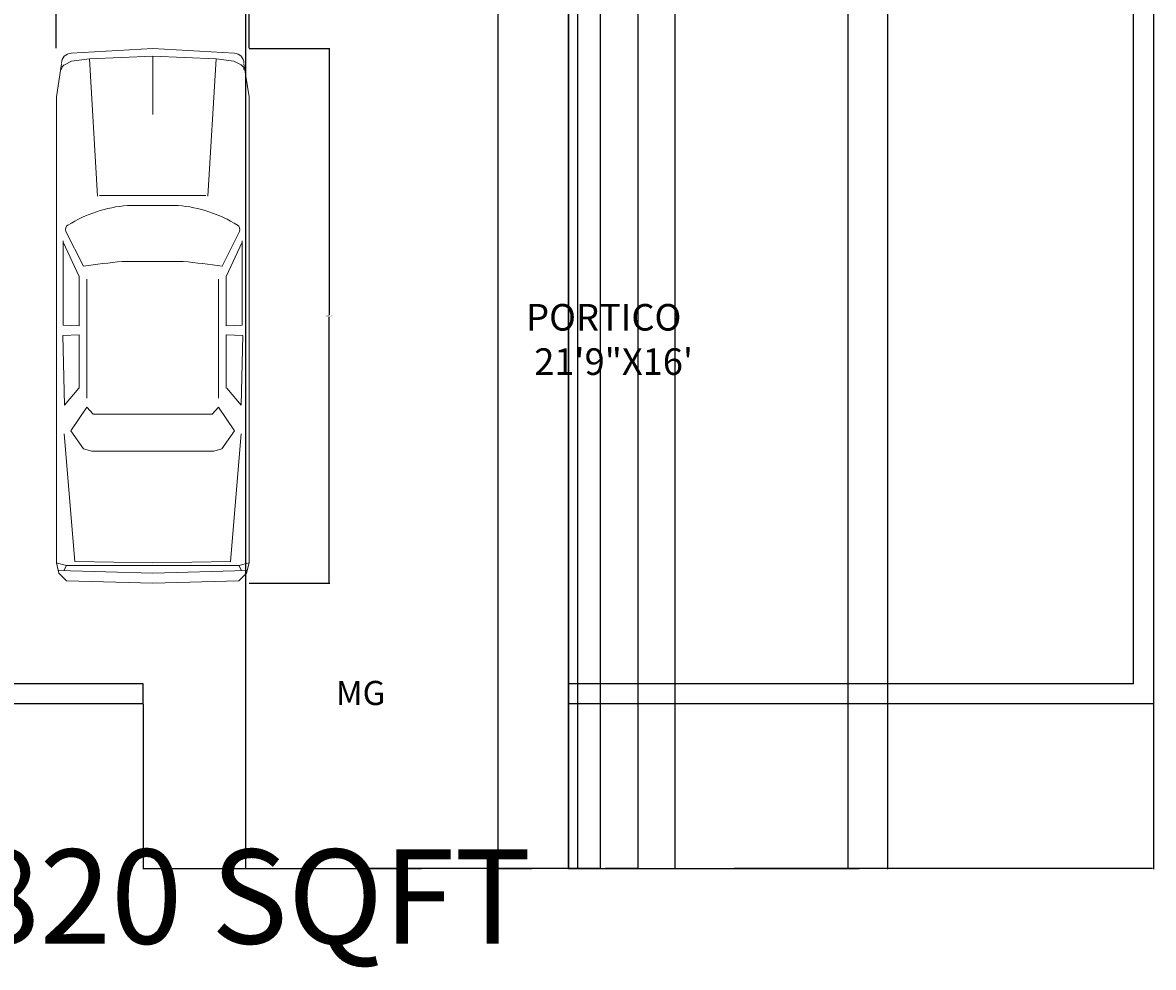
# Model space of a CAD drawing. Units: inches. Extents: x 503 to 1084, y -605 to 132.
# Tile 6 of 14: x 791 to 1046, y -605 to -392. Entities that reach past the tile are written whole.
import ezdxf

# ---------------------------------------------------------------- set-up
doc = ezdxf.new("R2010")
doc.units = ezdxf.units.IN
doc.header["$MEASUREMENT"] = 0
for name, color, linetype, lineweight in [('A-ANNO-DIMS', 7, 'Continuous', 18), ('A-ANNO-TEXT', 7, 'Continuous', 18), ('A-AREA-IDEN', 8, 'Continuous', 18), ('A-EQPM-VEHC', 50, 'Continuous', 13), ('C-PROP', 1, 'Continuous', 25)]:
    doc.layers.add(name, color=color, linetype=linetype, lineweight=lineweight)
doc.styles.get("Standard").update_dxf_attribs({"font": 'arial.ttf'})
doc.dimstyles.get("Standard").update_dxf_attribs({"dimtxt": 0.18, "dimasz": 0.18, "dimexe": 0.18, "dimexo": 0.0625, "dimgap": 0.09, "dimtad": 0, "dimtih": 1, "dimtoh": 1, "dimdec": 1, "dimzin": 0, "dimdsep": 46, "dimlunit": 4, "dimtxsty": 'Standard', "dimcen": 0.09, "dimadec": 0, "dimazin": 0, "dimtfac": 1, "dimtdec": 1, "dimtofl": 0, "dimtmove": 0, "dimatfit": 3, "dimfxl": 1, "dimtolj": 1, "dimtzin": 0, "dimarcsym": 0})

# ---------------------------------------------------------------- blocks, each defined once
blk = doc.blocks.new('02PCAR12')
at = {"color": 0, "linetype": 'ByBlock'}
for p, q in [((-207, 37), (-210, 34)), ((-203, 38), (-207, 37)), ((-206, 37), (-207, 0)), ((-203, 38.08), (-204, 34.08)), ((-19, 38), (-203, 38)), ((-6, 36), (-19, 38)), ((-210, 34), (-211, 0)), ((-204, 34.08), (-206, 35.08)), ((-204, -34), (-204, 34)), ((-202.36, 30.78), (-152, 35)), ((-150.83, 32.3), (-157.9, 27.3)), ((-141.48, 25.99), (-150.83, 32.3)), ((-113.23, 35.5), (-140.79, 34.89)), ((-140.79, 34.89), (-133.96, 29.23)), ((-113, 29), (-113.23, 35.5)), ((-109.42, 29.02), (-109.19, 35.33)), ((-109.19, 35.33), (-75.91, 35.3)), ((-76.45, 35.3), (-90, 29)), ((-72.15, 34.24), (-85.91, 27.37)), ((-5, 32), (-6.45, 34.89)), ((-5, 32), (-4, 25)), ((0, 0), (-1.8, 32.21)), ((-202.36, 30.78), (-203, 0)), ((-157.9, 27.3), (-158.93, 24.08)), ((-134, 29), (-113, 29)), ((-90, 29), (-109.42, 29.02)), ((-158.93, 24.08), (-158.93, -24)), ((-141.48, 25.99), (-144.24, 23.52)), ((-144.24, 23.52), (-144.24, 0)), ((-91, 26), (-138, 26)), ((-58.25, 21.76), (-4, 25)), ((-4, 25), (-3, 0)), ((-58, 0), (-58, 21)), ((-84, -12), (-84, 12)), ((-62, 10), (-62, 0)), ((-210, -34), (-211, 0)), ((-206, -37), (-207, 0)), ((-202.36, -30.78), (-203, 0)), ((-144.24, -23.52), (-144.24, 0)), ((-62, -10), (-62, 0)), ((-58, 0), (-58, -21)), ((-3, 0), (-26, 0)), ((-4, -25), (-3, 0)), ((0, 0), (-1.8, -32.21)), ((-58.25, -21.76), (-4, -25)), ((-157.9, -27.3), (-158.93, -24.08)), ((-141.48, -25.99), (-150.83, -32.3)), ((-141.48, -25.99), (-144.24, -23.52)), ((-91, -26), (-138, -26)), ((-5, -32), (-4, -25)), ((-202.36, -30.69), (-152, -34.92)), ((-150.83, -32.3), (-157.9, -27.3)), ((-140.79, -34.89), (-133.96, -29.23)), ((-134, -29), (-113, -29)), ((-113, -29), (-113.23, -35.5)), ((-90, -29), (-109.42, -29.02)), ((-109.42, -29.02), (-109.19, -35.33)), ((-76.45, -35.3), (-90, -29)), ((-72.15, -34.24), (-85.91, -27.37)), ((-207, -37), (-210, -34)), ((-204, -34), (-206, -35)), ((-203, -38), (-204, -34)), ((-113.23, -35.5), (-140.79, -34.89)), ((-109.19, -35.33), (-75.91, -35.3)), ((-5, -32), (-6.45, -34.89)), ((-203, -38), (-207, -37)), ((-19, -38), (-203, -38)), ((-6, -36), (-19, -38))]:
    blk.add_line(p, q, dxfattribs=at)
for centre, radius, start, end in [((-8.24, 34), 2, 26.5651, 90), ((-5.8, 32), 4, 3.0128, 90), ((-71.36, 32.4), 2, 31.5638, 113.1257), ((-115.33, 5.39), 53.61, 4.9379, 31.5638), ((-461.05, -27.14), 379.08, 5.9264, 8.267), ((-461.05, 27.14), 379.08, 351.733, 354.0736), ((-115.33, -5.39), 53.61, 328.4362, 355.0621), ((-71.36, -32.4), 2, 246.8743, 328.4362), ((-8.24, -34), 2, 270, 333.4349), ((-5.8, -32), 4, 270, 356.9872)]:
    blk.add_arc(centre, radius, start, end, dxfattribs=at)
blk = doc.blocks.new('*D36')
at = {"layer": 'A-ANNO-DIMS', "color": 0, "lineweight": -2, "transparency": 16777216}
for p, q in [((842.01, -397.95), (860.23, -397.95)), ((860.05, -398.13), (860.05, -458.1)), ((860.05, -518.43), (860.05, -458.46)), ((842.01, -518.61), (860.23, -518.61))]:
    blk.add_line(p, q, dxfattribs=at)
at = {"layer": 'A-ANNO-DIMS', "color": 0, "transparency": 16777216}
for points in [[(860.02, -398.13), (860.08, -398.13), (860.05, -397.95)], [(860.02, -518.43), (860.08, -518.43), (860.05, -518.61)]]:
    blk.add_solid(points, dxfattribs=at)
at = {"layer": 'Defpoints', "color": 0, "transparency": 16777216}
for p in [(841.95, -397.95), (860.05, -397.95), (841.95, -518.61)]:
    blk.add_point(p, dxfattribs=at)
at = {"layer": 'A-ANNO-DIMS', "color": 0, "transparency": 16777216, "insert": (860.05, -458.28), "char_height": 0.18, "attachment_point": 5}
blk.add_mtext('\\A1;CAR 10\'-0 1/2"', dxfattribs=at)
blk = doc.blocks.new('*D37')
at = {"layer": 'A-ANNO-DIMS', "color": 0, "lineweight": -2, "transparency": 16777216}
for p, q in [((798.44, -397.88), (798.44, -379.67)), ((798.62, -379.85), (819.65, -379.85)), ((841.77, -379.85), (820.73, -379.85)), ((841.95, -397.88), (841.95, -379.67))]:
    blk.add_line(p, q, dxfattribs=at)
at = {"layer": 'A-ANNO-DIMS', "color": 0, "transparency": 16777216}
for points in [[(798.62, -379.82), (798.62, -379.88), (798.44, -379.85)], [(841.77, -379.82), (841.77, -379.88), (841.95, -379.85)]]:
    blk.add_solid(points, dxfattribs=at)
at = {"layer": 'Defpoints', "color": 0, "transparency": 16777216}
for p in [(798.44, -379.85), (798.44, -397.95), (841.95, -397.95)]:
    blk.add_point(p, dxfattribs=at)
at = {"layer": 'A-ANNO-DIMS', "color": 0, "transparency": 16777216, "insert": (820.19, -379.85), "char_height": 0.18, "attachment_point": 5}
blk.add_mtext('\\A1;3\'-7 1/2"', dxfattribs=at)
blk = doc.blocks.new('*D38')
at = {"layer": 'A-ANNO-DIMS', "color": 0, "lineweight": -2, "transparency": 16777216}
for p, q in [((818.09, -545.88), (818.09, -583.15)), ((914.09, -545.88), (914.09, -583.15)), ((818.27, -582.97), (865.76, -582.97)), ((913.91, -582.97), (866.42, -582.97))]:
    blk.add_line(p, q, dxfattribs=at)
at = {"layer": 'A-ANNO-DIMS', "color": 0, "transparency": 16777216}
for points in [[(818.27, -582.94), (818.27, -583), (818.09, -582.97)], [(913.91, -582.94), (913.91, -583), (914.09, -582.97)]]:
    blk.add_solid(points, dxfattribs=at)
at = {"layer": 'Defpoints', "color": 0, "transparency": 16777216}
for p in [(818.09, -545.82), (914.09, -545.82), (914.09, -582.97)]:
    blk.add_point(p, dxfattribs=at)
at = {"layer": 'A-ANNO-DIMS', "color": 0, "transparency": 16777216, "insert": (866.09, -582.97), "char_height": 0.18, "attachment_point": 5}
blk.add_mtext('\\A1;8\'-0"', dxfattribs=at)
blk = doc.blocks.new('*D39')
at = {"layer": 'A-ANNO-DIMS', "color": 0, "lineweight": -2, "transparency": 16777216}
for p, q in [((914.09, -545.88), (914.09, -583.15)), ((1046.09, -545.88), (1046.09, -583.15)), ((914.27, -582.97), (979.7, -582.97)), ((1045.91, -582.97), (980.48, -582.97))]:
    blk.add_line(p, q, dxfattribs=at)
at = {"layer": 'A-ANNO-DIMS', "color": 0, "transparency": 16777216}
for points in [[(914.27, -582.94), (914.27, -583), (914.09, -582.97)], [(1045.91, -582.94), (1045.91, -583), (1046.09, -582.97)]]:
    blk.add_solid(points, dxfattribs=at)
at = {"layer": 'Defpoints', "color": 0, "transparency": 16777216}
for p in [(914.09, -545.82), (1046.09, -545.82), (1046.09, -582.97)]:
    blk.add_point(p, dxfattribs=at)
at = {"layer": 'A-ANNO-DIMS', "color": 0, "transparency": 16777216, "insert": (980.09, -582.97), "char_height": 0.18, "attachment_point": 5}
blk.add_mtext('\\A1;11\'-0"', dxfattribs=at)
blk = doc.blocks.new('*D47')
at = {"layer": 'A-ANNO-DIMS', "color": 0, "lineweight": -2, "transparency": 16777216}
for p, q in [((916.09, -363.88), (916.09, -583.15)), ((986.09, -363.88), (986.09, -583.15)), ((916.27, -582.97), (950.69, -582.97)), ((985.91, -582.97), (951.49, -582.97))]:
    blk.add_line(p, q, dxfattribs=at)
at = {"layer": 'A-ANNO-DIMS', "color": 0, "transparency": 16777216}
for points in [[(916.27, -582.94), (916.27, -583), (916.09, -582.97)], [(985.91, -582.94), (985.91, -583), (986.09, -582.97)]]:
    blk.add_solid(points, dxfattribs=at)
at = {"layer": 'Defpoints', "color": 0, "transparency": 16777216}
for p in [(916.09, -363.82), (986.09, -363.82), (986.09, -582.97)]:
    blk.add_point(p, dxfattribs=at)
at = {"layer": 'A-ANNO-DIMS', "color": 0, "transparency": 16777216, "insert": (951.09, -582.97), "char_height": 0.18, "attachment_point": 5}
blk.add_mtext('\\A1;5\'-10"', dxfattribs=at)
blk = doc.blocks.new('*D64')
at = {"layer": 'A-ANNO-DIMS', "color": 0, "lineweight": -2, "transparency": 16777216}
for p, q in [((938.09, -162.88), (938.09, -583.15)), ((977.09, -162.88), (977.09, -583.15)), ((938.27, -582.97), (957.26, -582.97)), ((976.91, -582.97), (957.92, -582.97))]:
    blk.add_line(p, q, dxfattribs=at)
at = {"layer": 'A-ANNO-DIMS', "color": 0, "transparency": 16777216}
for points in [[(938.27, -582.94), (938.27, -583), (938.09, -582.97)], [(976.91, -582.94), (976.91, -583), (977.09, -582.97)]]:
    blk.add_solid(points, dxfattribs=at)
at = {"layer": 'Defpoints', "color": 0, "transparency": 16777216}
for p in [(938.09, -162.82), (977.09, -162.82), (977.09, -582.97)]:
    blk.add_point(p, dxfattribs=at)
at = {"layer": 'A-ANNO-DIMS', "color": 0, "transparency": 16777216, "insert": (957.59, -582.97), "char_height": 0.18, "attachment_point": 5}
blk.add_mtext('\\A1;3\'-3"', dxfattribs=at)
blk = doc.blocks.new('*D65')
at = {"layer": 'A-ANNO-DIMS', "color": 0, "lineweight": -2, "transparency": 16777216}
for p, q in [((898.09, -162.88), (898.09, -583.15)), ((914.09, -162.88), (914.09, -583.15)), ((898.27, -582.97), (905.77, -582.97)), ((913.91, -582.97), (906.41, -582.97))]:
    blk.add_line(p, q, dxfattribs=at)
at = {"layer": 'A-ANNO-DIMS', "color": 0, "transparency": 16777216}
for points in [[(898.27, -582.94), (898.27, -583), (898.09, -582.97)], [(913.91, -582.94), (913.91, -583), (914.09, -582.97)]]:
    blk.add_solid(points, dxfattribs=at)
at = {"layer": 'Defpoints', "color": 0, "transparency": 16777216}
for p in [(898.09, -162.82), (914.09, -162.82), (914.09, -582.97)]:
    blk.add_point(p, dxfattribs=at)
at = {"layer": 'A-ANNO-DIMS', "color": 0, "transparency": 16777216, "insert": (906.09, -582.97), "char_height": 0.18, "attachment_point": 5}
blk.add_mtext('\\A1;1\'-4"', dxfattribs=at)
blk = doc.blocks.new('*D66')
at = {"layer": 'A-ANNO-DIMS', "color": 0, "lineweight": -2, "transparency": 16777216}
for p, q in [((841.16, -387.88), (841.16, -583.15)), ((921.2, -387.88), (921.2, -583.15)), ((841.34, -582.97), (880.85, -582.97)), ((921.02, -582.97), (881.51, -582.97))]:
    blk.add_line(p, q, dxfattribs=at)
at = {"layer": 'A-ANNO-DIMS', "color": 0, "transparency": 16777216}
for points in [[(841.34, -582.94), (841.34, -583), (841.16, -582.97)], [(921.02, -582.94), (921.02, -583), (921.2, -582.97)]]:
    blk.add_solid(points, dxfattribs=at)
at = {"layer": 'Defpoints', "color": 0, "transparency": 16777216}
for p in [(841.16, -387.82), (921.2, -387.82), (921.2, -582.97)]:
    blk.add_point(p, dxfattribs=at)
at = {"layer": 'A-ANNO-DIMS', "color": 0, "transparency": 16777216, "insert": (881.18, -582.97), "char_height": 0.18, "attachment_point": 5}
blk.add_mtext('\\A1;6\'-8"', dxfattribs=at)
blk = doc.blocks.new('*D78')
at = {"layer": 'A-ANNO-DIMS', "color": 0, "lineweight": -2, "transparency": 16777216}
for p, q in [((913.97, -276.31), (913.97, -583.15)), ((929.71, -276.31), (929.71, -583.15)), ((914.15, -582.97), (921.31, -582.97)), ((929.53, -582.97), (922.37, -582.97))]:
    blk.add_line(p, q, dxfattribs=at)
at = {"layer": 'A-ANNO-DIMS', "color": 0, "transparency": 16777216}
for points in [[(914.15, -582.94), (914.15, -583), (913.97, -582.97)], [(929.53, -582.94), (929.53, -583), (929.71, -582.97)]]:
    blk.add_solid(points, dxfattribs=at)
at = {"layer": 'Defpoints', "color": 0, "transparency": 16777216}
for p in [(913.97, -276.25), (929.71, -276.25), (929.71, -582.97)]:
    blk.add_point(p, dxfattribs=at)
at = {"layer": 'A-ANNO-DIMS', "color": 0, "transparency": 16777216, "insert": (921.84, -582.97), "char_height": 0.18, "attachment_point": 5}
blk.add_mtext('\\A1;1\'-3 1/2"', dxfattribs=at)

msp = doc.modelspace()

# ---------------------------------------------------------------- linework, layer by layer
at = {"layer": 'C-PROP'}
for p, q in [((1046.09, 6.18), (1046.09, -545.82)), ((1041.59, -541.32), (1041.59, 1.68)), ((818.09, -541.32), (594.59, -541.32)), ((818.09, -545.82), (818.09, -541.32)), ((1041.59, -541.32), (914.09, -541.32)), ((914.09, -545.82), (914.09, -541.32)), ((818.09, -545.82), (590.09, -545.82)), ((1046.09, -545.82), (914.09, -545.82))]:
    msp.add_line(p, q, dxfattribs=at)

# ---------------------------------------------------------------- block references
at = {"layer": 'A-EQPM-VEHC', "xscale": 0.5718767357715869, "yscale": 0.5718767357715869, "zscale": 0.5718767357715869, "rotation": 89.99999999999999}
msp.add_blockref('02PCAR12', (820.22, -397.95), dxfattribs=at)

# ---------------------------------------------------------------- texts
at = {"layer": 'A-ANNO-TEXT'}
msp.add_text('MG', height=5.444, dxfattribs=at).set_placement((861.57, -546.1))
at = {"layer": 'A-ANNO-TEXT', "insert": (675.5, -578.68), "char_height": 21.2807, "attachment_point": 1}
msp.add_mtext_dynamic_manual_height_columns('AREA=1820 SQFT', width=263.9184, gutter_width=3.55, heights=[0], dxfattribs=at)
at = {"layer": 'A-AREA-IDEN', "insert": (897.17, -455.6), "char_height": 6, "attachment_point": 1}
msp.add_mtext_dynamic_manual_height_columns('    PORTICO\\P     21\'9"X16\'', width=54.3765, gutter_width=1, heights=[0], dxfattribs=at)

# ---------------------------------------------------------------- dimensions: what is measured, and where the dimension line sits
at = {"layer": 'A-ANNO-DIMS'}
for base, p1, p2, picture, middle in [((914.09, -582.97), (898.09, -162.82), (914.09, -162.82), '*D65', (906.09, -582.97)), ((977.09, -582.97), (938.09, -162.82), (977.09, -162.82), '*D64', (957.59, -582.97)), ((929.71, -582.97), (913.97, -276.25), (929.71, -276.25), '*D78', (921.84, -582.97)), ((986.09, -582.97), (916.09, -363.82), (986.09, -363.82), '*D47', (951.09, -582.97)), ((921.2, -582.97), (841.16, -387.82), (921.2, -387.82), '*D66', (881.18, -582.97)), ((914.09, -582.97), (818.09, -545.82), (914.09, -545.82), '*D38', (866.09, -582.97)), ((1046.09, -582.97), (914.09, -545.82), (1046.09, -545.82), '*D39', (980.09, -582.97))]:
    dim = msp.add_linear_dim(base=base, p1=p1, p2=p2, dimstyle='Standard', override={"dimdec": 1, "dimlfac": 1, "dimrnd": 0, "dimzin": 1, "dimdsep": 46, "dimlunit": 4, "dimfrac": 2}, dxfattribs=at)
    dim.commit()
    dim.dimension.update_dxf_attribs({"geometry": picture, "text_midpoint": middle})
dim = msp.add_linear_dim(base=(798.44, -379.85), p1=(841.95, -397.95), p2=(798.44, -397.95), angle=180, dimstyle='Standard', override={"dimdec": 1, "dimlfac": 1, "dimrnd": 0, "dimzin": 1, "dimdsep": 46, "dimlunit": 4, "dimfrac": 2}, dxfattribs=at)
dim.commit()
dim.dimension.update_dxf_attribs({"geometry": '*D37', "text_midpoint": (820.19, -379.85)})
dim = msp.add_linear_dim(base=(860.05, -397.95), p1=(841.95, -518.61), p2=(841.95, -397.95), angle=90, text='CAR <>', dimstyle='Standard', override={"dimdec": 1, "dimlfac": 1, "dimrnd": 0, "dimzin": 1, "dimdsep": 46, "dimlunit": 4, "dimfrac": 2}, dxfattribs=at)
dim.commit()
dim.dimension.update_dxf_attribs({"geometry": '*D36', "text_midpoint": (860.05, -458.28)})

doc.saveas('drawing.dxf')
